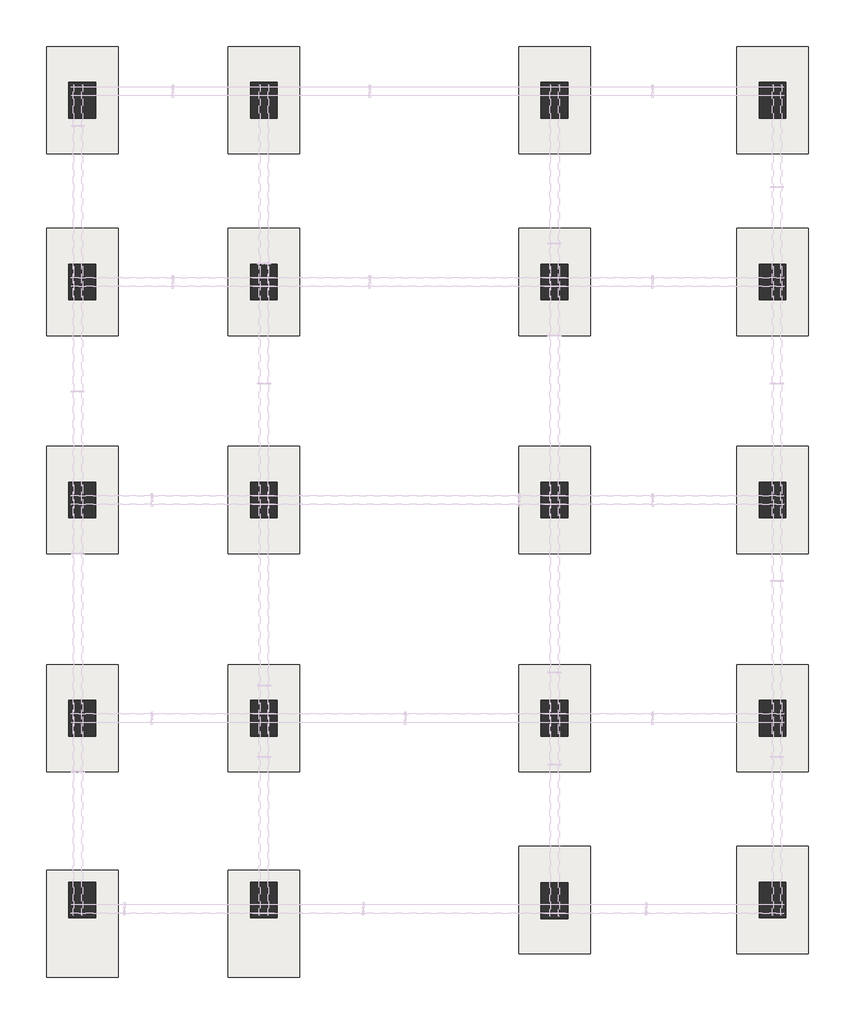
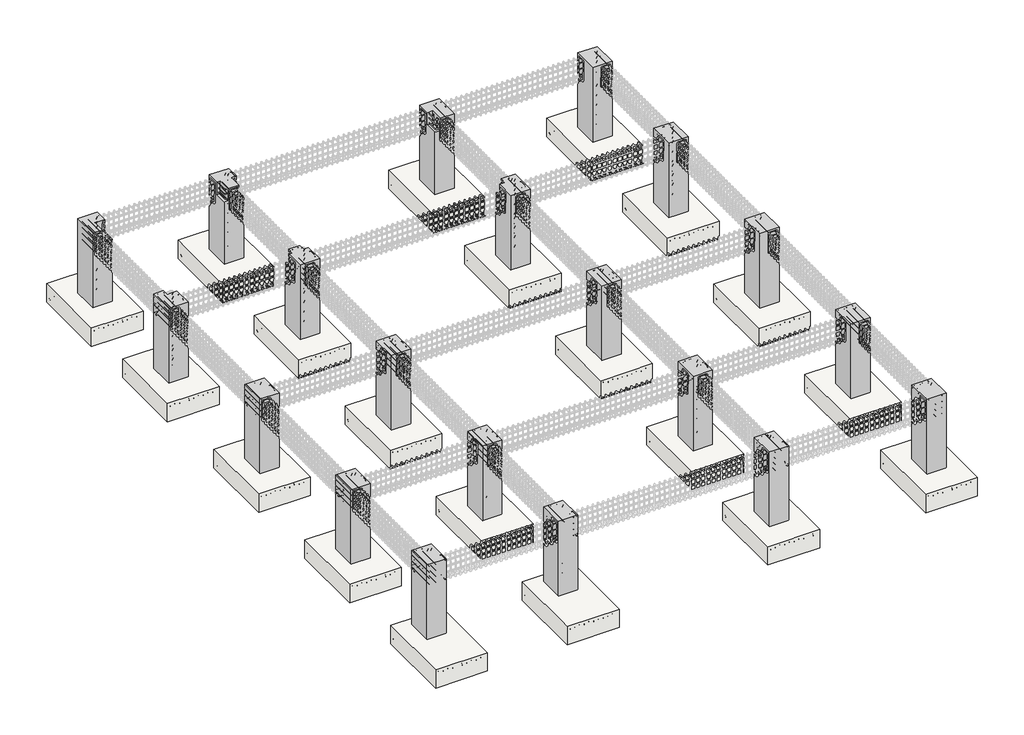
# One storey, part 1 of 16: 20 columns, 20 slabs.
"""IFC4 building model written with IfcOpenShell, lengths in millimetres."""

from ifc_helpers import new_model, si_unit, frame, origin, place, context, project, spatial, polyline, outline, extrude, faceted_brep, transform, mapped, element, save
from components import m_footing_rectangular_1800_x_1200_x_450mm_16ba7ea5

model = new_model("IFC4")

# Units and contexts
model_context = context("Model", 3, world=origin())
ifc_project = project(units=[si_unit("LENGTHUNIT", "METRE", prefix="MILLI")], contexts=[model_context])

# Site, building, storey
site = spatial("IfcSite", under=ifc_project)
building = spatial("IfcBuilding", under=site)
storey = spatial("IfcBuildingStorey", under=building, Elevation=-1828.8)

# Columns
placement = place(None, origin())
element("IfcColumn", 1, ObjectType="M_Concrete-Rectangular-Column : 450 x 600mm", at=placement, inside=storey, context=model_context, shape_type="Brep", body=[
    faceted_brep([(-5151.1302026, 12545.6151954, -1828.8), (-5151.1302026, 11945.6151954, -1828.8), (-5601.1302026, 11945.6151954, -1828.8), (-5601.1302026, 12545.6151954, -1828.8), (-5151.1302026, 12545.6151954, 0.0), (-5151.1302026, 12245.6151954, 0.0), (-5151.1302026, 12245.6151954, -300.0), (-5151.1302026, 11945.6151954, -300.0), (-5376.1302026, 11945.6151954, -300.0), (-5376.1302026, 11945.6151954, 0.0), (-5601.1302026, 11945.6151954, 0.0), (-5601.1302026, 12545.6151954, 0.0), (-5376.1302026, 12245.6151954, 0.0), (-5376.1302026, 12245.6151954, -300.0)], [[[0, 1, 2, 3]], [[1, 0, 4, 5, 6, 7]], [[2, 1, 7, 8, 9, 10]], [[3, 2, 10, 11]], [[0, 3, 11, 4]], [[11, 10, 9, 12, 5, 4]], [[6, 13, 8, 7]], [[13, 12, 9, 8]], [[12, 13, 6, 5]]]),
])
element("IfcColumn", 2, ObjectType="M_Concrete-Rectangular-Column : 450 x 600mm", at=placement, inside=storey, context=model_context, shape_type="Brep", body=[
    faceted_brep([(-2103.1302026, 12545.6151954, -1828.8), (-2103.1302026, 11945.6151954, -1828.8), (-2553.1302026, 11945.6151954, -1828.8), (-2553.1302026, 12545.6151954, -1828.8), (-2103.1302026, 12545.6151954, 0.0), (-2103.1302026, 12245.6151954, 0.0), (-2103.1302026, 12245.6151954, -300.0), (-2103.1302026, 11945.6151954, -300.0), (-2216.0245126, 11945.6151954, -300.0), (-2216.0245126, 11945.6151954, 0.0), (-2476.1302026, 11945.6151954, 0.0), (-2476.1302026, 11945.6151954, -300.0), (-2553.1302026, 11945.6151954, -300.0), (-2553.1302026, 12245.6151954, -300.0), (-2553.1302026, 12245.6151954, 0.0), (-2553.1302026, 12545.6151954, 0.0), (-2476.1302026, 12245.6151954, 0.0), (-2216.0245126, 12245.6151954, 0.0), (-2216.0245126, 12245.6151954, -300.0), (-2476.1302026, 12245.6151954, -300.0)], [[[0, 1, 2, 3]], [[1, 0, 4, 5, 6, 7]], [[2, 1, 7, 8, 9, 10, 11, 12]], [[3, 2, 12, 13, 14, 15]], [[0, 3, 15, 4]], [[4, 15, 14, 16, 10, 9, 17, 5]], [[6, 18, 8, 7]], [[16, 19, 11, 10]], [[19, 16, 14, 13]], [[18, 17, 9, 8]], [[17, 18, 6, 5]], [[19, 13, 12, 11]]]),
])
element("IfcColumn", 3, ObjectType="M_Concrete-Rectangular-Column : 450 x 600mm", at=placement, inside=storey, context=model_context, shape_type="Brep", body=[
    faceted_brep([(2773.6697974, 12545.6151954, -1828.8), (2773.6697974, 11945.6151954, -1828.8), (2323.6697974, 11945.6151954, -1828.8), (2323.6697974, 12545.6151954, -1828.8), (2773.6697974, 12545.6151954, 0.0), (2773.6697974, 11945.6151954, 0.0), (2448.4912316, 11945.6151954, 0.0), (2448.4912316, 11945.6151954, -300.0), (2323.6697974, 11945.6151954, -300.0), (2323.6697974, 12245.6151954, -300.0), (2323.6697974, 12245.6151954, 0.0), (2323.6697974, 12545.6151954, 0.0), (2448.4912316, 12245.6151954, 0.0), (2448.4912316, 12245.6151954, -300.0)], [[[0, 1, 2, 3]], [[1, 0, 4, 5]], [[2, 1, 5, 6, 7, 8]], [[3, 2, 8, 9, 10, 11]], [[0, 3, 11, 4]], [[5, 4, 11, 10, 12, 6]], [[7, 13, 9, 8]], [[13, 12, 10, 9]], [[12, 13, 7, 6]]]),
])
element("IfcColumn", 4, ObjectType="M_Concrete-Rectangular-Column : 450 x 600mm", at=placement, inside=storey, context=model_context, shape_type="SweptSolid", body=[
    extrude(outline(polyline([(6431.2697974, 12545.6151954), (6431.2697974, 11945.6151954), (5981.2697974, 11945.6151954), (5981.2697974, 12545.6151954), (6431.2697974, 12545.6151954)])), frame((0.0, 0.0, -1828.8), z_axis=(0.0, 0.0, 1.0), x_axis=(1.0, 0.0, 0.0)), (0.0, 0.0, 1.0), 1828.8),
])
element("IfcColumn", 5, ObjectType="M_Concrete-Rectangular-Column : 450 x 600mm", at=placement, inside=storey, context=model_context, shape_type="Brep", body=[
    faceted_brep([(-5151.1302026, 9497.6151954, -1828.8), (-5151.1302026, 8897.6151954, -1828.8), (-5601.1302026, 8897.6151954, -1828.8), (-5601.1302026, 9497.6151954, -1828.8), (-5151.1302026, 9497.6151954, -300.0), (-5151.1302026, 9345.6151954, -300.0), (-5151.1302026, 9345.6151954, 0.0), (-5151.1302026, 8897.6151954, 0.0), (-5601.1302026, 8897.6151954, 0.0), (-5601.1302026, 9497.6151954, 0.0), (-5376.1302026, 9497.6151954, 0.0), (-5376.1302026, 9497.6151954, -300.0), (-5376.1302026, 9345.6151954, 0.0), (-5376.1302026, 9345.6151954, -300.0)], [[[0, 1, 2, 3]], [[1, 0, 4, 5, 6, 7]], [[2, 1, 7, 8]], [[3, 2, 8, 9]], [[0, 3, 9, 10, 11, 4]], [[8, 7, 6, 12, 10, 9]], [[11, 13, 5, 4]], [[13, 12, 6, 5]], [[12, 13, 11, 10]]]),
])
element("IfcColumn", 6, ObjectType="M_Concrete-Rectangular-Column : 450 x 600mm", at=placement, inside=storey, context=model_context, shape_type="Brep", body=[
    faceted_brep([(-2103.1302026, 9497.6151954, -1828.8), (-2103.1302026, 8897.6151954, -1828.8), (-2553.1302026, 8897.6151954, -1828.8), (-2553.1302026, 9497.6151954, -1828.8), (-2103.1302026, 9497.6151954, -300.0), (-2103.1302026, 9345.6151954, -300.0), (-2103.1302026, 9345.6151954, 0.0), (-2103.1302026, 8897.6151954, 0.0), (-2553.1302026, 8897.6151954, 0.0), (-2553.1302026, 9345.6151954, 0.0), (-2553.1302026, 9345.6151954, -300.0), (-2553.1302026, 9497.6151954, -300.0), (-2476.1302026, 9497.6151954, -300.0), (-2476.1302026, 9497.6151954, 0.0), (-2216.0245126, 9497.6151954, 0.0), (-2216.0245126, 9497.6151954, -300.0), (-2216.0245126, 9345.6151954, 0.0), (-2476.1302026, 9345.6151954, 0.0), (-2216.0245126, 9345.6151954, -300.0), (-2476.1302026, 9345.6151954, -300.0)], [[[0, 1, 2, 3]], [[1, 0, 4, 5, 6, 7]], [[2, 1, 7, 8]], [[3, 2, 8, 9, 10, 11]], [[0, 3, 11, 12, 13, 14, 15, 4]], [[8, 7, 6, 16, 14, 13, 17, 9]], [[18, 5, 4, 15]], [[19, 17, 13, 12]], [[17, 19, 10, 9]], [[16, 18, 15, 14]], [[18, 16, 6, 5]], [[10, 19, 12, 11]]]),
])
element("IfcColumn", 7, ObjectType="M_Concrete-Rectangular-Column : 450 x 600mm", at=placement, inside=storey, context=model_context, shape_type="Brep", body=[
    faceted_brep([(2773.6697974, 9497.6151954, -1828.8), (2773.6697974, 8897.6151954, -1828.8), (2323.6697974, 8897.6151954, -1828.8), (2323.6697974, 9497.6151954, -1828.8), (2773.6697974, 9497.6151954, 0.0), (2773.6697974, 8897.6151954, 0.0), (2323.6697974, 8897.6151954, 0.0), (2323.6697974, 9345.6151954, 0.0), (2323.6697974, 9345.6151954, -300.0), (2323.6697974, 9497.6151954, -300.0), (2448.4912316, 9497.6151954, -300.0), (2448.4912316, 9497.6151954, 0.0), (2448.4912316, 9345.6151954, 0.0), (2448.4912316, 9345.6151954, -300.0)], [[[0, 1, 2, 3]], [[1, 0, 4, 5]], [[2, 1, 5, 6]], [[3, 2, 6, 7, 8, 9]], [[0, 3, 9, 10, 11, 4]], [[5, 4, 11, 12, 7, 6]], [[8, 13, 10, 9]], [[13, 12, 11, 10]], [[12, 13, 8, 7]]]),
])
element("IfcColumn", 8, ObjectType="M_Concrete-Rectangular-Column : 450 x 600mm", at=placement, inside=storey, context=model_context, shape_type="SweptSolid", body=[
    extrude(outline(polyline([(6431.2697974, 9497.6151954), (6431.2697974, 8897.6151954), (5981.2697974, 8897.6151954), (5981.2697974, 9497.6151954), (6431.2697974, 9497.6151954)])), frame((0.0, 0.0, -1828.8), z_axis=(0.0, 0.0, 1.0), x_axis=(1.0, 0.0, 0.0)), (0.0, 0.0, 1.0), 1828.8),
])
element("IfcColumn", 9, ObjectType="M_Concrete-Rectangular-Column : 450 x 600mm", at=placement, inside=storey, context=model_context, shape_type="SweptSolid", body=[
    extrude(outline(polyline([(-5151.1302026, 5840.0151954), (-5151.1302026, 5240.0151954), (-5601.1302026, 5240.0151954), (-5601.1302026, 5840.0151954), (-5151.1302026, 5840.0151954)])), frame((0.0, 0.0, -1828.8), z_axis=(0.0, 0.0, 1.0), x_axis=(1.0, 0.0, 0.0)), (0.0, 0.0, 1.0), 1828.8),
])
element("IfcColumn", 10, ObjectType="M_Concrete-Rectangular-Column : 450 x 600mm", at=placement, inside=storey, context=model_context, shape_type="SweptSolid", body=[
    extrude(outline(polyline([(-2103.1302026, 5840.0151954), (-2103.1302026, 5240.0151954), (-2553.1302026, 5240.0151954), (-2553.1302026, 5840.0151954), (-2103.1302026, 5840.0151954)])), frame((0.0, 0.0, -1828.8), z_axis=(0.0, 0.0, 1.0), x_axis=(1.0, 0.0, 0.0)), (0.0, 0.0, 1.0), 1828.8),
])
element("IfcColumn", 11, ObjectType="M_Concrete-Rectangular-Column : 450 x 600mm", at=placement, inside=storey, context=model_context, shape_type="SweptSolid", body=[
    extrude(outline(polyline([(2773.6697974, 5840.0151954), (2773.6697974, 5240.0151954), (2323.6697974, 5240.0151954), (2323.6697974, 5840.0151954), (2773.6697974, 5840.0151954)])), frame((0.0, 0.0, -1828.8), z_axis=(0.0, 0.0, 1.0), x_axis=(1.0, 0.0, 0.0)), (0.0, 0.0, 1.0), 1828.8),
])
element("IfcColumn", 12, ObjectType="M_Concrete-Rectangular-Column : 450 x 600mm", at=placement, inside=storey, context=model_context, shape_type="SweptSolid", body=[
    extrude(outline(polyline([(6431.2697974, 5840.0151954), (6431.2697974, 5240.0151954), (5981.2697974, 5240.0151954), (5981.2697974, 5840.0151954), (6431.2697974, 5840.0151954)])), frame((0.0, 0.0, -1828.8), z_axis=(0.0, 0.0, 1.0), x_axis=(1.0, 0.0, 0.0)), (0.0, 0.0, 1.0), 1828.8),
])
element("IfcColumn", 13, ObjectType="M_Concrete-Rectangular-Column : 450 x 600mm", at=placement, inside=storey, context=model_context, shape_type="SweptSolid", body=[
    extrude(outline(polyline([(6431.2697974, 2182.4151954), (6431.2697974, 1582.4151954), (5981.2697974, 1582.4151954), (5981.2697974, 2182.4151954), (6431.2697974, 2182.4151954)])), frame((0.0, 0.0, -1828.8), z_axis=(0.0, 0.0, 1.0), x_axis=(1.0, 0.0, 0.0)), (0.0, 0.0, 1.0), 1828.8),
])
element("IfcColumn", 14, ObjectType="M_Concrete-Rectangular-Column : 450 x 600mm", at=placement, inside=storey, context=model_context, shape_type="SweptSolid", body=[
    extrude(outline(polyline([(2773.6697974, 2182.4151954), (2773.6697974, 1582.4151954), (2323.6697974, 1582.4151954), (2323.6697974, 2182.4151954), (2773.6697974, 2182.4151954)])), frame((0.0, 0.0, -1828.8), z_axis=(0.0, 0.0, 1.0), x_axis=(1.0, 0.0, 0.0)), (0.0, 0.0, 1.0), 1828.8),
])
element("IfcColumn", 15, ObjectType="M_Concrete-Rectangular-Column : 450 x 600mm", at=placement, inside=storey, context=model_context, shape_type="SweptSolid", body=[
    extrude(outline(polyline([(-2103.1302026, 2182.4151954), (-2103.1302026, 1582.4151954), (-2553.1302026, 1582.4151954), (-2553.1302026, 2182.4151954), (-2103.1302026, 2182.4151954)])), frame((0.0, 0.0, -1828.8), z_axis=(0.0, 0.0, 1.0), x_axis=(1.0, 0.0, 0.0)), (0.0, 0.0, 1.0), 1828.8),
])
element("IfcColumn", 16, ObjectType="M_Concrete-Rectangular-Column : 450 x 600mm", at=placement, inside=storey, context=model_context, shape_type="SweptSolid", body=[
    extrude(outline(polyline([(-5151.1302026, 2182.4151954), (-5151.1302026, 1582.4151954), (-5601.1302026, 1582.4151954), (-5601.1302026, 2182.4151954), (-5151.1302026, 2182.4151954)])), frame((0.0, 0.0, -1828.8), z_axis=(0.0, 0.0, 1.0), x_axis=(1.0, 0.0, 0.0)), (0.0, 0.0, 1.0), 1828.8),
])
element("IfcColumn", 17, ObjectType="M_Concrete-Rectangular-Column : 450 x 600mm", at=placement, inside=storey, context=model_context, shape_type="SweptSolid", body=[
    extrude(outline(polyline([(-5151.1302026, -865.5848046), (-5151.1302026, -1465.5848046), (-5601.1302026, -1465.5848046), (-5601.1302026, -865.5848046), (-5151.1302026, -865.5848046)])), frame((0.0, 0.0, -1828.8), z_axis=(0.0, 0.0, 1.0), x_axis=(1.0, 0.0, 0.0)), (0.0, 0.0, 1.0), 1828.8),
])
element("IfcColumn", 18, ObjectType="M_Concrete-Rectangular-Column : 450 x 600mm", at=placement, inside=storey, context=model_context, shape_type="SweptSolid", body=[
    extrude(outline(polyline([(-2103.1302026, -865.5848046), (-2103.1302026, -1465.5848046), (-2553.1302026, -1465.5848046), (-2553.1302026, -865.5848046), (-2103.1302026, -865.5848046)])), frame((0.0, 0.0, -1828.8), z_axis=(0.0, 0.0, 1.0), x_axis=(1.0, 0.0, 0.0)), (0.0, 0.0, 1.0), 1828.8),
])
element("IfcColumn", 19, ObjectType="M_Concrete-Rectangular-Column : 450 x 600mm", at=placement, inside=storey, context=model_context, shape_type="SweptSolid", body=[
    extrude(outline(polyline([(2773.6697974, -877.5848046), (2773.6697974, -1477.5848046), (2323.6697974, -1477.5848046), (2323.6697974, -877.5848046), (2773.6697974, -877.5848046)])), frame((0.0, 0.0, -1828.8), z_axis=(0.0, 0.0, 1.0), x_axis=(1.0, 0.0, 0.0)), (0.0, 0.0, 1.0), 1828.8),
])
element("IfcColumn", 20, ObjectType="M_Concrete-Rectangular-Column : 450 x 600mm", at=placement, inside=storey, context=model_context, shape_type="SweptSolid", body=[
    extrude(outline(polyline([(6431.2697974, -865.5848046), (6431.2697974, -1465.5848046), (5981.2697974, -1465.5848046), (5981.2697974, -865.5848046), (6431.2697974, -865.5848046)])), frame((0.0, 0.0, -1828.8), z_axis=(0.0, 0.0, 1.0), x_axis=(1.0, 0.0, 0.0)), (0.0, 0.0, 1.0), 1828.8),
])

# Slabs
m_footing_rectangular_1800_x_1200_x_450mm_shape = m_footing_rectangular_1800_x_1200_x_450mm_16ba7ea5(model_context)
element("IfcSlab", 21, ObjectType="M_Footing-Rectangular : 1800 x 1200 x 450mm", at=placement, inside=storey, context=model_context, shape_type="MappedRepresentation", body=[
    mapped(m_footing_rectangular_1800_x_1200_x_450mm_shape, transform((-5376.1302026, 12245.6151954, -1828.8), x_axis=(1.0, 0.0, 0.0), y_axis=(0.0, 1.0, 0.0), z_axis=(0.0, 0.0, 1.0))),
])
element("IfcSlab", 22, ObjectType="M_Footing-Rectangular : 1800 x 1200 x 450mm", at=placement, inside=storey, context=model_context, shape_type="MappedRepresentation", body=[
    mapped(m_footing_rectangular_1800_x_1200_x_450mm_shape, transform((-2328.1302026, 12245.6151954, -1828.8), x_axis=(1.0, 0.0, 0.0), y_axis=(0.0, 1.0, 0.0), z_axis=(0.0, 0.0, 1.0))),
])
element("IfcSlab", 23, ObjectType="M_Footing-Rectangular : 1800 x 1200 x 450mm", at=placement, inside=storey, context=model_context, shape_type="MappedRepresentation", body=[
    mapped(m_footing_rectangular_1800_x_1200_x_450mm_shape, transform((2548.6697974, 12245.6151954, -1828.8), x_axis=(1.0, 0.0, 0.0), y_axis=(0.0, 1.0, 0.0), z_axis=(0.0, 0.0, 1.0))),
])
element("IfcSlab", 24, ObjectType="M_Footing-Rectangular : 1800 x 1200 x 450mm", at=placement, inside=storey, context=model_context, shape_type="MappedRepresentation", body=[
    mapped(m_footing_rectangular_1800_x_1200_x_450mm_shape, transform((6206.2697974, 12245.6151954, -1828.8), x_axis=(1.0, 0.0, 0.0), y_axis=(0.0, 1.0, 0.0), z_axis=(0.0, 0.0, 1.0))),
])
element("IfcSlab", 25, ObjectType="M_Footing-Rectangular : 1800 x 1200 x 450mm", at=placement, inside=storey, context=model_context, shape_type="MappedRepresentation", body=[
    mapped(m_footing_rectangular_1800_x_1200_x_450mm_shape, transform((-5376.1302026, 9197.6151954, -1828.8), x_axis=(1.0, 0.0, 0.0), y_axis=(0.0, 1.0, 0.0), z_axis=(0.0, 0.0, 1.0))),
])
element("IfcSlab", 26, ObjectType="M_Footing-Rectangular : 1800 x 1200 x 450mm", at=placement, inside=storey, context=model_context, shape_type="MappedRepresentation", body=[
    mapped(m_footing_rectangular_1800_x_1200_x_450mm_shape, transform((-2328.1302026, 9197.6151954, -1828.8), x_axis=(1.0, 0.0, 0.0), y_axis=(0.0, 1.0, 0.0), z_axis=(0.0, 0.0, 1.0))),
])
element("IfcSlab", 27, ObjectType="M_Footing-Rectangular : 1800 x 1200 x 450mm", at=placement, inside=storey, context=model_context, shape_type="MappedRepresentation", body=[
    mapped(m_footing_rectangular_1800_x_1200_x_450mm_shape, transform((2548.6697974, 9197.6151954, -1828.8), x_axis=(1.0, 0.0, 0.0), y_axis=(0.0, 1.0, 0.0), z_axis=(0.0, 0.0, 1.0))),
])
element("IfcSlab", 28, ObjectType="M_Footing-Rectangular : 1800 x 1200 x 450mm", at=placement, inside=storey, context=model_context, shape_type="MappedRepresentation", body=[
    mapped(m_footing_rectangular_1800_x_1200_x_450mm_shape, transform((6206.2697974, 9197.6151954, -1828.8), x_axis=(1.0, 0.0, 0.0), y_axis=(0.0, 1.0, 0.0), z_axis=(0.0, 0.0, 1.0))),
])
element("IfcSlab", 29, ObjectType="M_Footing-Rectangular : 1800 x 1200 x 450mm", at=placement, inside=storey, context=model_context, shape_type="MappedRepresentation", body=[
    mapped(m_footing_rectangular_1800_x_1200_x_450mm_shape, transform((6206.2697974, 5540.0151954, -1828.8), x_axis=(1.0, 0.0, 0.0), y_axis=(0.0, 1.0, 0.0), z_axis=(0.0, 0.0, 1.0))),
])
element("IfcSlab", 30, ObjectType="M_Footing-Rectangular : 1800 x 1200 x 450mm", at=placement, inside=storey, context=model_context, shape_type="MappedRepresentation", body=[
    mapped(m_footing_rectangular_1800_x_1200_x_450mm_shape, transform((2548.6697974, 5540.0151954, -1828.8), x_axis=(1.0, 0.0, 0.0), y_axis=(0.0, 1.0, 0.0), z_axis=(0.0, 0.0, 1.0))),
])
element("IfcSlab", 31, ObjectType="M_Footing-Rectangular : 1800 x 1200 x 450mm", at=placement, inside=storey, context=model_context, shape_type="MappedRepresentation", body=[
    mapped(m_footing_rectangular_1800_x_1200_x_450mm_shape, transform((-2328.1302026, 5540.0151954, -1828.8), x_axis=(1.0, 0.0, 0.0), y_axis=(0.0, 1.0, 0.0), z_axis=(0.0, 0.0, 1.0))),
])
element("IfcSlab", 32, ObjectType="M_Footing-Rectangular : 1800 x 1200 x 450mm", at=placement, inside=storey, context=model_context, shape_type="MappedRepresentation", body=[
    mapped(m_footing_rectangular_1800_x_1200_x_450mm_shape, transform((-5376.1302026, 5540.0151954, -1828.8), x_axis=(1.0, 0.0, 0.0), y_axis=(0.0, 1.0, 0.0), z_axis=(0.0, 0.0, 1.0))),
])
element("IfcSlab", 33, ObjectType="M_Footing-Rectangular : 1800 x 1200 x 450mm", at=placement, inside=storey, context=model_context, shape_type="MappedRepresentation", body=[
    mapped(m_footing_rectangular_1800_x_1200_x_450mm_shape, transform((-5376.1302026, 1882.4151954, -1828.8), x_axis=(1.0, 0.0, 0.0), y_axis=(0.0, 1.0, 0.0), z_axis=(0.0, 0.0, 1.0))),
])
element("IfcSlab", 34, ObjectType="M_Footing-Rectangular : 1800 x 1200 x 450mm", at=placement, inside=storey, context=model_context, shape_type="MappedRepresentation", body=[
    mapped(m_footing_rectangular_1800_x_1200_x_450mm_shape, transform((-2328.1302026, 1882.4151954, -1828.8), x_axis=(1.0, 0.0, 0.0), y_axis=(0.0, 1.0, 0.0), z_axis=(0.0, 0.0, 1.0))),
])
element("IfcSlab", 35, ObjectType="M_Footing-Rectangular : 1800 x 1200 x 450mm", at=placement, inside=storey, context=model_context, shape_type="MappedRepresentation", body=[
    mapped(m_footing_rectangular_1800_x_1200_x_450mm_shape, transform((2548.6697974, 1882.4151954, -1828.8), x_axis=(1.0, 0.0, 0.0), y_axis=(0.0, 1.0, 0.0), z_axis=(0.0, 0.0, 1.0))),
])
element("IfcSlab", 36, ObjectType="M_Footing-Rectangular : 1800 x 1200 x 450mm", at=placement, inside=storey, context=model_context, shape_type="MappedRepresentation", body=[
    mapped(m_footing_rectangular_1800_x_1200_x_450mm_shape, transform((6206.2697974, 1882.4151954, -1828.8), x_axis=(1.0, 0.0, 0.0), y_axis=(0.0, 1.0, 0.0), z_axis=(0.0, 0.0, 1.0))),
])
element("IfcSlab", 37, ObjectType="M_Footing-Rectangular : 1800 x 1200 x 450mm", at=placement, inside=storey, context=model_context, shape_type="MappedRepresentation", body=[
    mapped(m_footing_rectangular_1800_x_1200_x_450mm_shape, transform((6206.2697974, -1165.5848046, -1828.8), x_axis=(1.0, 0.0, 0.0), y_axis=(0.0, 1.0, 0.0), z_axis=(0.0, 0.0, 1.0))),
])
element("IfcSlab", 38, ObjectType="M_Footing-Rectangular : 1800 x 1200 x 450mm", at=placement, inside=storey, context=model_context, shape_type="MappedRepresentation", body=[
    mapped(m_footing_rectangular_1800_x_1200_x_450mm_shape, transform((2548.6697974, -1165.5848046, -1828.8), x_axis=(1.0, 0.0, 0.0), y_axis=(0.0, 1.0, 0.0), z_axis=(0.0, 0.0, 1.0))),
])
element("IfcSlab", 39, ObjectType="M_Footing-Rectangular : 1800 x 1200 x 450mm", at=placement, inside=storey, context=model_context, shape_type="MappedRepresentation", body=[
    mapped(m_footing_rectangular_1800_x_1200_x_450mm_shape, transform((-2328.1302026, -1565.5848046, -1828.8), x_axis=(1.0, 0.0, 0.0), y_axis=(0.0, 1.0, 0.0), z_axis=(0.0, 0.0, 1.0))),
])
element("IfcSlab", 40, ObjectType="M_Footing-Rectangular : 1800 x 1200 x 450mm", at=placement, inside=storey, context=model_context, shape_type="MappedRepresentation", body=[
    mapped(m_footing_rectangular_1800_x_1200_x_450mm_shape, transform((-5376.1302026, -1565.5848046, -1828.8), x_axis=(1.0, 0.0, 0.0), y_axis=(0.0, 1.0, 0.0), z_axis=(0.0, 0.0, 1.0))),
])

save(model, "model.ifc")

# Revit data of these elements
# Grids (mm)
#   "E": line (10076.762, 1882.415) -> (-6395.576, 1882.415)
#   "1": line (-5376.13, 14612.802) -> (-5376.13, -5102.337)
#   "2": line (-2328.13, 14612.802) -> (-2328.13, -5102.337)
#   "3": line (2548.67, 14612.802) -> (2548.67, -5102.337)
#   "4": line (6206.27, 14612.802) -> (6206.27, -5102.337)
#   "A": line (10076.762, 12245.615) -> (-6395.576, 12245.615)
#   "B": line (10076.762, 9197.615) -> (-6395.576, 9197.615)
#   "D": line (10076.762, 5540.015) -> (-6395.576, 5540.015)
#   "F": line (10076.762, -1165.585) -> (-6395.576, -1165.585)
# Type "M_Concrete-Rectangular-Column : 450 x 600mm"
#   b = 1' - 5.71654"
#   h = 1' - 11.62205"
#   Structural Material [instance default] = Concrete, Cast-in-Place gray
# Type "M_Footing-Rectangular : 1800 x 1200 x 450mm"
#   Width = 3' - 11.24409"
#   Length = 5' - 10.86614"
#   Foundation Thickness = 1' - 5.71654"
#   Structural Material [instance default] = Concrete, Cast-in-Place gray
#   Assembly Code = ""
# Elements 1, 2, 3, 4, 5, 6, 7, 8, 9, 10, 11, 12, 13, 14, 15, 16, 17, 18, 19, 20 (IfcColumn, "M_Concrete-Rectangular-Column : 450 x 600mm")
#   Structural Material = Concrete, Cast-in-Place gray
#   Phase Created = New Construction
#   Materials on its faces: "Concrete, Cast-in-Place gray"
# Elements 21, 22, 23, 24, 25, 26, 27, 28, 29, 30, 31, 32, 33, 34, 35, 36, 37, 38, 39, 40 (IfcSlab, "M_Footing-Rectangular : 1800 x 1200 x 450mm")
#   Structural Material = Concrete, Cast-in-Place gray
#   Phase Created = New Construction
#   Materials on its faces: "Concrete, Cast-in-Place gray"
# Materials
#   "Concrete, Cast-in-Place gray": class "Concrete", colour RGB 192 192 192, transparency 0, Description = "Cast-in-place concrete", Cost = 0
